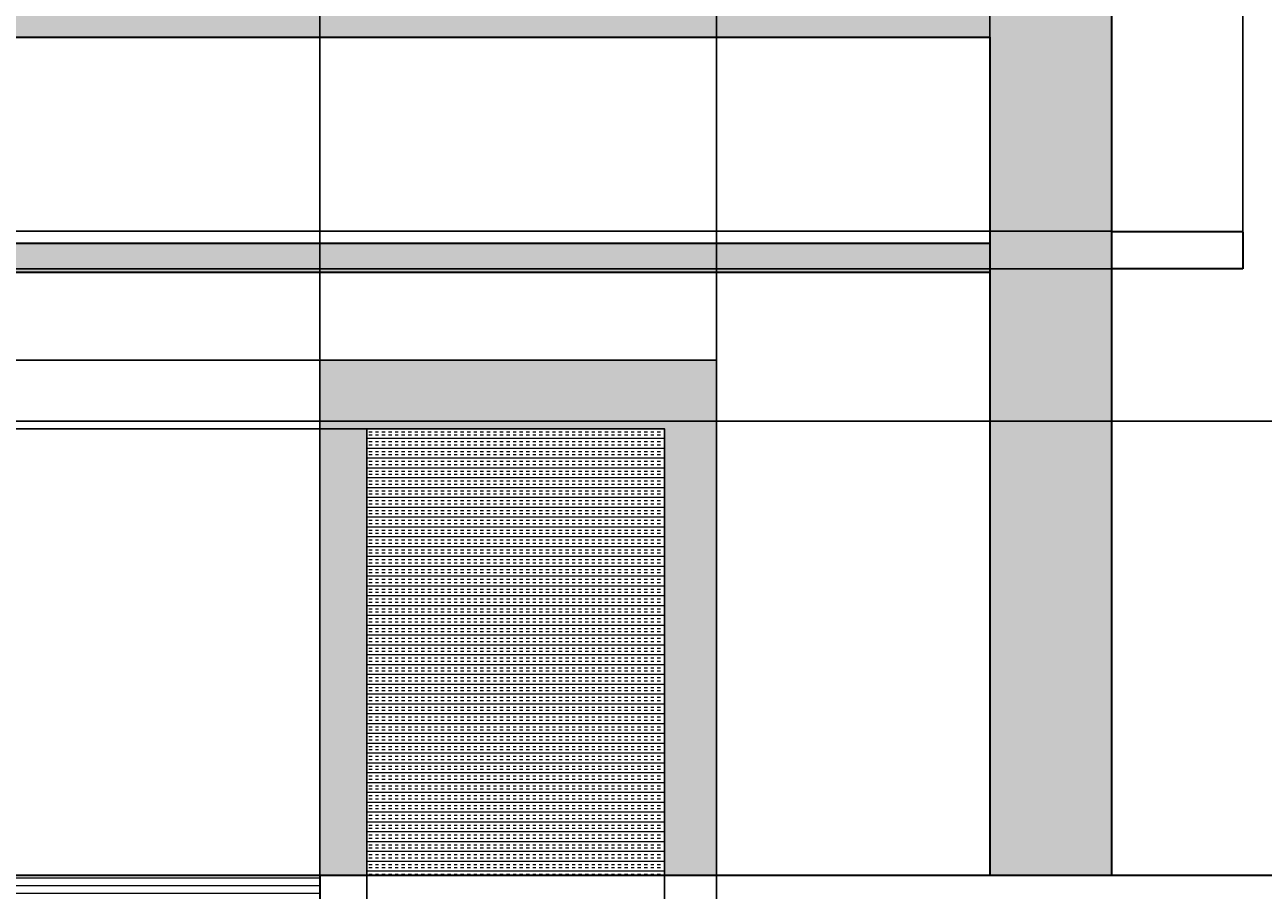
# Model space of a CAD drawing. Units: inches. Extents: x -5 to 714, y 84 to 644.
# Tile 16 of 20: x 457 to 613, y 199 to 308. Entities that reach past the tile are written whole.
import ezdxf

# ---------------------------------------------------------------- set-up
doc = ezdxf.new("R2010")
doc.units = ezdxf.units.IN
doc.header["$MEASUREMENT"] = 0
for name, color, linetype, lineweight in [('A-ANNO-DIMS', 2, 'Continuous', 18), ('A-DOOR', 4, 'Continuous', 25), ('A-ELEV', 7, 'Continuous', 35), ('A-ELEV-PATT', 8, 'Continuous', 13)]:
    doc.layers.add(name, color=color, linetype=linetype, lineweight=lineweight)
doc.styles.get("Standard").update_dxf_attribs({"font": 'arial.ttf'})
doc.dimstyles.get("Standard").update_dxf_attribs({"dimtxt": 0.9375, "dimasz": 0.18, "dimexe": 0.18, "dimexo": 0.0625, "dimgap": 0.09, "dimtad": 0, "dimtih": 1, "dimtoh": 1, "dimdec": 4, "dimzin": 0, "dimdsep": 46, "dimlunit": 4, "dimtxsty": 'Standard', "dimcen": 0.09, "dimadec": 0, "dimazin": 0, "dimtfac": 1, "dimtdec": 4, "dimtofl": 0, "dimtmove": 0, "dimatfit": 3, "dimfxl": 1, "dimtolj": 1, "dimtzin": 0, "dimarcsym": 0})

# ---------------------------------------------------------------- blocks, each defined once
blk = doc.blocks.new('*D55')
at = {"layer": 'A-ANNO-DIMS', "color": 0, "lineweight": -2, "transparency": 16777216}
for p, q in [((593.49, 315.1), (712.66, 315.1)), ((712.48, 314.92), (712.48, 258.71)), ((712.48, 201.37), (712.48, 257.58)), ((593.49, 201.19), (712.66, 201.19))]:
    blk.add_line(p, q, dxfattribs=at)
at = {"layer": 'A-ANNO-DIMS', "color": 0, "transparency": 16777216}
for points in [[(712.45, 314.92), (712.51, 314.92), (712.48, 315.1)], [(712.45, 201.37), (712.51, 201.37), (712.48, 201.19)]]:
    blk.add_solid(points, dxfattribs=at)
at = {"layer": 'Defpoints', "color": 0, "transparency": 16777216}
for p in [(593.43, 315.1), (712.48, 315.1), (593.43, 201.19)]:
    blk.add_point(p, dxfattribs=at)
at = {"layer": 'A-ANNO-DIMS', "color": 0, "transparency": 16777216, "insert": (712.48, 258.14), "char_height": 0.938, "attachment_point": 5}
blk.add_mtext('\\A1;113.9', dxfattribs=at)
blk = doc.blocks.new('*D56')
at = {"layer": 'A-ANNO-DIMS', "color": 0, "lineweight": -2, "transparency": 16777216}
for p, q in [((578.03, 277.05), (-2.74, 277.05)), ((-2.56, 276.87), (-2.56, 239.69)), ((-2.56, 201.37), (-2.56, 238.55)), ((578.03, 201.19), (-2.74, 201.19))]:
    blk.add_line(p, q, dxfattribs=at)
at = {"layer": 'A-ANNO-DIMS', "color": 0, "transparency": 16777216}
for points in [[(-2.59, 276.87), (-2.53, 276.87), (-2.56, 277.05)], [(-2.59, 201.37), (-2.53, 201.37), (-2.56, 201.19)]]:
    blk.add_solid(points, dxfattribs=at)
at = {"layer": 'Defpoints', "color": 0, "transparency": 16777216}
for p in [(-2.56, 277.05), (578.09, 277.05), (578.09, 201.19)]:
    blk.add_point(p, dxfattribs=at)
at = {"layer": 'A-ANNO-DIMS', "color": 0, "transparency": 16777216, "insert": (-2.56, 239.12), "char_height": 0.938, "attachment_point": 5}
blk.add_mtext('\\A1;75.86', dxfattribs=at)
blk = doc.blocks.new('*D57')
at = {"layer": 'A-ANNO-DIMS', "color": 0, "lineweight": -2, "transparency": 16777216}
for p, q in [((578.03, 306.63), (-2.74, 306.63)), ((-2.56, 306.45), (-2.56, 292.41)), ((-2.56, 277.23), (-2.56, 291.27)), ((578.03, 277.05), (-2.74, 277.05))]:
    blk.add_line(p, q, dxfattribs=at)
at = {"layer": 'A-ANNO-DIMS', "color": 0, "transparency": 16777216}
for points in [[(-2.59, 306.45), (-2.53, 306.45), (-2.56, 306.63)], [(-2.59, 277.23), (-2.53, 277.23), (-2.56, 277.05)]]:
    blk.add_solid(points, dxfattribs=at)
at = {"layer": 'Defpoints', "color": 0, "transparency": 16777216}
for p in [(578.09, 306.63), (-2.56, 277.05), (578.09, 277.05)]:
    blk.add_point(p, dxfattribs=at)
at = {"layer": 'A-ANNO-DIMS', "color": 0, "transparency": 16777216, "insert": (-2.56, 291.84), "char_height": 0.938, "attachment_point": 5}
blk.add_mtext('\\A1;29.58', dxfattribs=at)
blk = doc.blocks.new('*D58')
at = {"layer": 'A-ANNO-DIMS', "color": 0, "lineweight": -2, "transparency": 16777216}
for p, q in [((593.43, 282.26), (593.43, 643.61)), ((593.61, 643.43), (600.15, 643.43)), ((609.76, 643.43), (603.22, 643.43)), ((609.94, 282.26), (609.94, 643.61))]:
    blk.add_line(p, q, dxfattribs=at)
at = {"layer": 'A-ANNO-DIMS', "color": 0, "transparency": 16777216}
for points in [[(593.61, 643.46), (593.61, 643.4), (593.43, 643.43)], [(609.76, 643.46), (609.76, 643.4), (609.94, 643.43)]]:
    blk.add_solid(points, dxfattribs=at)
at = {"layer": 'Defpoints', "color": 0, "transparency": 16777216}
for p in [(609.94, 643.43), (593.43, 282.2), (609.94, 282.2)]:
    blk.add_point(p, dxfattribs=at)
at = {"layer": 'A-ANNO-DIMS', "color": 0, "transparency": 16777216, "insert": (601.68, 643.43), "char_height": 0.938, "attachment_point": 5}
blk.add_mtext('\\A1;16.51', dxfattribs=at)
blk = doc.blocks.new('*D59')
at = {"layer": 'A-ANNO-DIMS', "color": 0, "lineweight": -2, "transparency": 16777216}
for p, q in [((593.37, 282.2), (-2.74, 282.2)), ((-2.56, 282.02), (-2.56, 280.41)), ((-2.56, 277.66), (-2.56, 279.27)), ((593.37, 277.48), (-2.74, 277.48))]:
    blk.add_line(p, q, dxfattribs=at)
at = {"layer": 'A-ANNO-DIMS', "color": 0, "transparency": 16777216}
for points in [[(-2.59, 282.02), (-2.53, 282.02), (-2.56, 282.2)], [(-2.59, 277.66), (-2.53, 277.66), (-2.56, 277.48)]]:
    blk.add_solid(points, dxfattribs=at)
at = {"layer": 'Defpoints', "color": 0, "transparency": 16777216}
for p in [(-2.56, 282.2), (593.43, 282.2), (593.43, 277.48)]:
    blk.add_point(p, dxfattribs=at)
at = {"layer": 'A-ANNO-DIMS', "color": 0, "transparency": 16777216, "insert": (-2.56, 279.84), "char_height": 0.938, "attachment_point": 5}
blk.add_mtext('\\A1;4.719', dxfattribs=at)
blk = doc.blocks.new('*D62')
at = {"layer": 'A-ANNO-DIMS', "color": 0, "lineweight": -2, "transparency": 16777216}
for p, q in [((407.38, 266.06), (407.38, 643.61)), ((407.56, 643.43), (449.27, 643.43)), ((493.6, 643.43), (451.89, 643.43)), ((493.78, 266.06), (493.78, 643.61))]:
    blk.add_line(p, q, dxfattribs=at)
at = {"layer": 'A-ANNO-DIMS', "color": 0, "transparency": 16777216}
for points in [[(407.56, 643.46), (407.56, 643.4), (407.38, 643.43)], [(493.6, 643.46), (493.6, 643.4), (493.78, 643.43)]]:
    blk.add_solid(points, dxfattribs=at)
at = {"layer": 'Defpoints', "color": 0, "transparency": 16777216}
for p in [(493.78, 643.43), (407.38, 266), (493.78, 266)]:
    blk.add_point(p, dxfattribs=at)
at = {"layer": 'A-ANNO-DIMS', "color": 0, "transparency": 16777216, "insert": (450.58, 643.43), "char_height": 0.938, "attachment_point": 5}
blk.add_mtext('\\A1;86.4', dxfattribs=at)
blk = doc.blocks.new('*D63')
at = {"layer": 'A-ANNO-DIMS', "color": 0, "lineweight": -2, "transparency": 16777216}
for p, q in [((493.78, 266.06), (493.78, 643.61)), ((493.96, 643.43), (517.06, 643.43)), ((543.54, 643.43), (520.44, 643.43)), ((543.72, 266.06), (543.72, 643.61))]:
    blk.add_line(p, q, dxfattribs=at)
at = {"layer": 'A-ANNO-DIMS', "color": 0, "transparency": 16777216}
for points in [[(493.96, 643.46), (493.96, 643.4), (493.78, 643.43)], [(543.54, 643.46), (543.54, 643.4), (543.72, 643.43)]]:
    blk.add_solid(points, dxfattribs=at)
at = {"layer": 'Defpoints', "color": 0, "transparency": 16777216}
for p in [(543.72, 643.43), (493.78, 266), (543.72, 266)]:
    blk.add_point(p, dxfattribs=at)
at = {"layer": 'A-ANNO-DIMS', "color": 0, "transparency": 16777216, "insert": (518.75, 643.43), "char_height": 0.938, "attachment_point": 5}
blk.add_mtext('\\A1;49.94', dxfattribs=at)
blk = doc.blocks.new('*D64')
at = {"layer": 'A-ANNO-DIMS', "color": 0, "lineweight": -2, "transparency": 16777216}
for p, q in [((543.72, 266.06), (543.72, 643.61)), ((543.9, 643.43), (558.86, 643.43)), ((577.91, 643.43), (562.94, 643.43)), ((578.09, 277.11), (578.09, 643.61))]:
    blk.add_line(p, q, dxfattribs=at)
at = {"layer": 'A-ANNO-DIMS', "color": 0, "transparency": 16777216}
for points in [[(543.9, 643.46), (543.9, 643.4), (543.72, 643.43)], [(577.91, 643.46), (577.91, 643.4), (578.09, 643.43)]]:
    blk.add_solid(points, dxfattribs=at)
at = {"layer": 'Defpoints', "color": 0, "transparency": 16777216}
for p in [(578.09, 643.43), (578.09, 277.05), (543.72, 266)]:
    blk.add_point(p, dxfattribs=at)
at = {"layer": 'A-ANNO-DIMS', "color": 0, "transparency": 16777216, "insert": (560.9, 643.43), "char_height": 0.938, "attachment_point": 5}
blk.add_mtext('\\A1;34.375', dxfattribs=at)
blk = doc.blocks.new('*D69')
at = {"layer": 'A-ANNO-DIMS', "color": 0, "lineweight": -2, "transparency": 16777216}
for p, q in [((403.5, 258.29), (712.66, 258.29)), ((712.48, 258.11), (712.48, 216.52)), ((712.48, 173.8), (712.48, 215.38)), ((403.5, 173.62), (712.66, 173.62))]:
    blk.add_line(p, q, dxfattribs=at)
at = {"layer": 'A-ANNO-DIMS', "color": 0, "transparency": 16777216}
for points in [[(712.45, 258.11), (712.51, 258.11), (712.48, 258.29)], [(712.45, 173.8), (712.51, 173.8), (712.48, 173.62)]]:
    blk.add_solid(points, dxfattribs=at)
at = {"layer": 'Defpoints', "color": 0, "transparency": 16777216}
for p in [(403.44, 258.29), (712.48, 258.29), (403.44, 173.62)]:
    blk.add_point(p, dxfattribs=at)
at = {"layer": 'A-ANNO-DIMS', "color": 0, "transparency": 16777216, "insert": (712.48, 215.95), "char_height": 0.938, "attachment_point": 5}
blk.add_mtext('\\A1;84.67', dxfattribs=at)
blk = doc.blocks.new('*D70')
at = {"layer": 'A-ANNO-DIMS', "color": 0, "lineweight": -2, "transparency": 16777216}
for p, q in [((499.68, 257.28), (499.68, 84.31)), ((537.18, 257.28), (537.18, 84.31)), ((499.86, 84.49), (517.12, 84.49)), ((537, 84.49), (519.74, 84.49))]:
    blk.add_line(p, q, dxfattribs=at)
at = {"layer": 'A-ANNO-DIMS', "color": 0, "transparency": 16777216}
for points in [[(499.86, 84.52), (499.86, 84.46), (499.68, 84.49)], [(537, 84.52), (537, 84.46), (537.18, 84.49)]]:
    blk.add_solid(points, dxfattribs=at)
at = {"layer": 'Defpoints', "color": 0, "transparency": 16777216}
for p in [(499.68, 257.34), (537.18, 257.34), (537.18, 84.49)]:
    blk.add_point(p, dxfattribs=at)
at = {"layer": 'A-ANNO-DIMS', "color": 0, "transparency": 16777216, "insert": (518.43, 84.49), "char_height": 0.938, "attachment_point": 5}
blk.add_mtext('\\A1;37.5', dxfattribs=at)
blk = doc.blocks.new('*D71')
at = {"layer": 'A-ANNO-DIMS', "color": 0, "lineweight": -2, "transparency": 16777216}
for p, q in [((537.12, 257.34), (-2.74, 257.34)), ((-2.56, 257.16), (-2.56, 229.83)), ((-2.56, 201.37), (-2.56, 228.7)), ((537.12, 201.19), (-2.74, 201.19))]:
    blk.add_line(p, q, dxfattribs=at)
at = {"layer": 'A-ANNO-DIMS', "color": 0, "transparency": 16777216}
for points in [[(-2.59, 257.16), (-2.53, 257.16), (-2.56, 257.34)], [(-2.59, 201.37), (-2.53, 201.37), (-2.56, 201.19)]]:
    blk.add_solid(points, dxfattribs=at)
at = {"layer": 'Defpoints', "color": 0, "transparency": 16777216}
for p in [(-2.56, 257.34), (537.18, 257.34), (537.18, 201.19)]:
    blk.add_point(p, dxfattribs=at)
at = {"layer": 'A-ANNO-DIMS', "color": 0, "transparency": 16777216, "insert": (-2.56, 229.27), "char_height": 0.938, "attachment_point": 5}
blk.add_mtext('\\A1;56.15', dxfattribs=at)
blk = doc.blocks.new('*D72')
at = {"layer": 'A-ANNO-DIMS', "color": 0, "lineweight": -2, "transparency": 16777216}
for p, q in [((493.71, 266), (-2.74, 266)), ((-2.56, 265.82), (-2.56, 234.17)), ((-2.56, 201.37), (-2.56, 233.03)), ((493.71, 201.19), (-2.74, 201.19))]:
    blk.add_line(p, q, dxfattribs=at)
at = {"layer": 'A-ANNO-DIMS', "color": 0, "transparency": 16777216}
for points in [[(-2.59, 265.82), (-2.53, 265.82), (-2.56, 266)], [(-2.59, 201.37), (-2.53, 201.37), (-2.56, 201.19)]]:
    blk.add_solid(points, dxfattribs=at)
at = {"layer": 'Defpoints', "color": 0, "transparency": 16777216}
for p in [(-2.56, 266), (493.78, 266), (493.78, 201.19)]:
    blk.add_point(p, dxfattribs=at)
at = {"layer": 'A-ANNO-DIMS', "color": 0, "transparency": 16777216, "insert": (-2.56, 233.6), "char_height": 0.938, "attachment_point": 5}
blk.add_mtext('\\A1;64.81', dxfattribs=at)

msp = doc.modelspace()

# ---------------------------------------------------------------- hatches: boundary and pattern name
at = {"layer": 'A-ELEV-PATT', "transparency": 33554687}
h = msp.add_hatch(color=256, dxfattribs=at)
h.dxf.hatch_style = 1
h.paths.add_polyline_path([(188.3677, 525.1928), (67.9893, 525.1928), (67.9893, 489.1928), (67.9893, 345.1928), (126.7303, 345.1928), (126.7303, 480.1709), (229.3575, 480.1709), (229.3575, 525.1928), (212.6043, 525.1928), (212.6043, 482.7164), (211.0019, 482.7164), (211.0019, 525.1928), (207.6919, 525.1928), (199.9852, 525.1928), (199.9852, 482.7164), (198.3828, 482.7164), (198.3828, 525.1928), (189.9701, 525.1928), (189.9701, 482.7164), (188.3677, 482.7164)])
h.paths.add_polyline_path([(121.3589, 336.2066), (75.5048, 336.2066), (75.5048, 319.345), (121.3589, 319.345)])
h.paths.add_polyline_path([(121.3589, 319.345), (75.5048, 319.345), (75.5048, 302.3045), (121.3589, 302.3045)])
h.paths.add_polyline_path([(121.3589, 302.3045), (75.5048, 302.3045), (75.5048, 282.8561), (121.3589, 282.8561)])
h.paths.add_polyline_path([(121.3589, 282.8561), (75.5048, 282.8561), (75.5048, 261.5556), (121.3589, 261.5556)])
h.paths.add_polyline_path([(121.3589, 261.5556), (75.5048, 261.5556), (75.5048, 243.7009), (121.3589, 243.7009)])
h.paths.add_polyline_path([(121.3589, 243.7009), (75.5048, 243.7009), (75.5048, 223.5117), (121.3589, 223.5117)])
h.paths.add_polyline_path([(121.3589, 223.5117), (75.5048, 223.5117), (75.5048, 212.5836), (121.3589, 212.5836)])
h.paths.add_polyline_path([(121.3589, 212.5836), (75.5048, 212.5836), (75.5048, 201.1928), (121.3589, 201.1928)])
h.paths.add_polyline_path([(179.9335, 201.1928), (30.1395, 201.1928), (30.1395, 198.7054), (179.9335, 198.7054)])
h.paths.add_polyline_path([(187.6349, 201.1928), (179.9335, 201.1928), (179.9335, 198.7054), (179.9335, 141.1928), (269.2446, 141.1928), (269.2446, 201.1928), (263.4349, 201.1928), (263.4349, 152.1176), (187.6349, 152.1176)])
h.paths.add_polyline_path([(269.2446, 277.0513), (269.2446, 287.501), (269.2446, 306.6286), (578.0915, 306.6286), (578.0915, 201.1928), (593.428, 201.1928), (593.428, 315.0968), (584.4202, 315.0968), (259.0665, 315.0968), (259.0665, 201.1928), (263.4349, 201.1928), (269.2446, 201.1928)])
h = msp.add_hatch(color=256, dxfattribs=at)
h.dxf.hatch_style = 1
h.paths.add_polyline_path([(289.8815, 417.0908), (237.2654, 417.0908), (237.2654, 345.1928), (289.8815, 345.1928)])
h.paths.add_polyline_path([(286.8815, 414.0908), (286.8815, 348.1928), (240.2654, 348.1928), (240.2654, 414.0908)], flags=16)
h.paths.add_polyline_path([(244.2856, 376.3091, -1), (241.2767, 376.3091, -1)], flags=0)
h.paths.add_polyline_path([(543.7164, 266.0021), (493.7771, 266.0021), (493.7771, 201.1928), (499.6809, 201.1928), (499.6809, 257.3379), (537.1779, 257.3379), (537.1779, 201.1928), (543.7164, 201.1928)])
h = msp.add_hatch(color=256, dxfattribs=at)
h.dxf.hatch_style = 1
h.paths.add_polyline_path([(578.0915, 280.7123), (269.2446, 280.7123), (269.2446, 277.0513), (578.0915, 277.0513)])
h = msp.add_hatch(color=256, dxfattribs=at)
h.dxf.hatch_style = 1
h.paths.add_polyline_path([(499.6809, 257.3379), (537.1779, 257.3379), (537.1779, 201.1928), (543.7164, 201.1928), (543.7164, 266.0021), (493.7771, 266.0021), (493.7771, 201.1928), (499.6809, 201.1928)])
h.paths.add_polyline_path([(407.3813, 197.3754), (403.4391, 197.3754), (403.4391, 191.3028), (407.3813, 191.3028)])
h.paths.add_polyline_path([(407.3813, 189.3028), (403.4391, 189.3028), (403.4391, 184.8307), (407.3813, 184.8307)])
h.paths.add_polyline_path([(407.3813, 182.8307), (403.4391, 182.8307), (403.4391, 177.6504), (407.3813, 177.6504)])
h.paths.add_polyline_path([(407.3813, 175.6504), (403.4391, 175.6504), (403.4391, 173.6169), (382.4961, 173.6169), (382.4961, 175.6504), (380.7784, 175.6504), (380.7784, 171.1197), (407.3813, 171.1197)])
h.paths.add_polyline_path([(382.4961, 182.8307), (380.7784, 182.8307), (380.7784, 177.6504), (382.4961, 177.6504)])
h.paths.add_polyline_path([(382.4961, 189.3028), (380.7784, 189.3028), (380.7784, 184.8307), (382.4961, 184.8307)])
h.paths.add_polyline_path([(382.4961, 197.3754), (380.7784, 197.3754), (380.7784, 191.3028), (382.4961, 191.3028)])
h.paths.add_polyline_path([(357.6527, 197.3754), (352.9482, 197.3754), (352.9482, 191.3028), (357.6527, 191.3028)])
h.paths.add_polyline_path([(357.6527, 189.3028), (352.9482, 189.3028), (352.9482, 184.8307), (357.6527, 184.8307)])
h.paths.add_polyline_path([(357.6527, 182.8307), (352.9482, 182.8307), (352.9482, 177.6504), (357.6527, 177.6504)])
h.paths.add_polyline_path([(376.2796, 173.6169), (357.6527, 173.6169), (357.6527, 175.6504), (352.9482, 175.6504), (352.9482, 173.6169), (343.9704, 173.6169), (343.9704, 171.1197), (376.2796, 171.1197)])
h.paths.add_polyline_path([(339.2672, 173.6169), (332.0052, 173.6169), (332.0052, 175.6504), (325.8305, 175.6504), (325.8305, 171.1197), (339.2672, 171.1197)])
h.paths.add_polyline_path([(332.0052, 182.8307), (325.8305, 182.8307), (325.8305, 177.6504), (332.0052, 177.6504)])
h.paths.add_polyline_path([(332.0052, 189.3028), (325.8305, 189.3028), (325.8305, 184.8307), (332.0052, 184.8307)])
h.paths.add_polyline_path([(332.0052, 197.3754), (325.8305, 197.3754), (325.8305, 191.3028), (332.0052, 191.3028)])
h = msp.add_hatch(dxfattribs=at)
h.set_pattern_fill('INSUL', color=256, scale=3.3)
h.paths.add_polyline_path([(537.1779, 257.3379), (499.6809, 257.3379), (499.6809, 201.1928), (537.1779, 201.1928)])
h = msp.add_hatch(dxfattribs=at)
h.set_pattern_fill('ANSI31', color=256, scale=7.8, angle=135)
h.paths.add_polyline_path([(493.7771, 201.1928), (454.6437, 201.1928), (454.6437, 141.1928), (493.7771, 141.1928)])
h.paths.add_polyline_path([(489.8003, 196.771), (489.8003, 143.3813), (458.6583, 143.3813), (458.6583, 196.771)], flags=16)

# ---------------------------------------------------------------- linework, layer by layer
at = {"layer": 'A-DOOR'}
for points in [[(493.7771, 266.0021), (543.7164, 266.0021), (543.7164, 158.7212), (493.7771, 158.7212)], [(499.6809, 257.3379), (537.1779, 257.3379), (537.1779, 201.1928), (499.6809, 201.1928)], [(493.7771, 201.1928), (543.7164, 201.1928), (543.7164, 141.1928), (493.7771, 141.1928)]]:
    msp.add_lwpolyline(points, close=True, dxfattribs=at)
at = {"layer": 'A-ELEV'}
for p, q in [((593.428, 315.0968), (593.428, 201.1928)), ((269.2446, 306.6286), (578.0915, 306.6286)), ((578.0915, 306.6286), (578.0915, 201.1928)), ((593.428, 282.1969), (609.9384, 282.1969)), ((609.9384, 282.1969), (609.9384, 277.4776)), ((269.2446, 280.7123), (578.0915, 280.7123)), ((609.9384, 277.4776), (593.428, 277.4776)), ((269.2446, 277.0513), (578.0915, 277.0513)), ((30.1395, 201.1928), (545.1065, 201.1928)), ((493.7771, 201.1928), (493.7771, 141.1928)), ((545.1065, 201.1928), (679.7826, 201.1928))]:
    msp.add_line(p, q, dxfattribs=at)

# ---------------------------------------------------------------- dimensions: what is measured, and where the dimension line sits
at = {"layer": 'A-ANNO-DIMS'}
for base, p1, p2, override, picture, middle in [((493.7771, 643.4276), (407.3813, 266.0021), (493.7771, 266.0021), {"dimdec": 1, "dimlfac": 1, "dimrnd": 0, "dimzin": 0, "dimdsep": 46, "dimlunit": 2}, '*D62', (450.5792, 643.4276)), ((543.7164, 643.4276), (493.7771, 266.0021), (543.7164, 266.0021), {"dimdec": 2, "dimlfac": 1, "dimrnd": 0, "dimzin": 0, "dimdsep": 46, "dimlunit": 2}, '*D63', (518.7468, 643.4276)), ((578.0915, 643.4276), (543.7164, 266.0021), (578.0915, 277.0513), {"dimdec": 3, "dimlfac": 1, "dimrnd": 0, "dimzin": 0, "dimdsep": 46, "dimlunit": 2}, '*D64', (560.904, 643.4276)), ((609.9384, 643.4276), (593.428, 282.1969), (609.9384, 282.1969), {"dimdec": 2, "dimlfac": 1, "dimrnd": 0, "dimzin": 0, "dimdsep": 46, "dimlunit": 2}, '*D58', (601.6832, 643.4276)), ((537.1779, 84.4928), (499.6809, 257.3379), (537.1779, 257.3379), {"dimdec": 1, "dimlfac": 1, "dimrnd": 0, "dimzin": 0, "dimdsep": 46, "dimlunit": 2}, '*D70', (518.4294, 84.4928))]:
    dim = msp.add_linear_dim(base=base, p1=p1, p2=p2, dimstyle='Standard', override=override, dxfattribs=at)
    dim.commit()
    dim.dimension.update_dxf_attribs({"geometry": picture, "text_midpoint": middle})
for base, p1, p2, override, picture, middle in [((712.4826, 315.0968), (593.428, 201.1928), (593.428, 315.0968), {"dimdec": 1, "dimlfac": 1, "dimrnd": 0, "dimzin": 0, "dimdsep": 46, "dimlunit": 2}, '*D55', (712.4826, 258.1448)), ((-2.5605, 277.0513), (578.0915, 306.6286), (578.0915, 277.0513), {"dimdec": 2, "dimlfac": 1, "dimrnd": 0, "dimzin": 0, "dimdsep": 46, "dimlunit": 2}, '*D57', (-2.5605, 291.84)), ((-2.5605, 282.1969), (593.428, 277.4776), (593.428, 282.1969), {"dimdec": 3, "dimlfac": 1, "dimrnd": 0, "dimzin": 0, "dimdsep": 46, "dimlunit": 2}, '*D59', (-2.5605, 279.8372)), ((-2.5605, 277.0513), (578.0915, 201.1928), (578.0915, 277.0513), {"dimdec": 2, "dimlfac": 1, "dimrnd": 0, "dimzin": 0, "dimdsep": 46, "dimlunit": 2}, '*D56', (-2.5605, 239.1221)), ((-2.5605, 266.0021), (493.7771, 201.1928), (493.7771, 266.0021), {"dimdec": 2, "dimlfac": 1, "dimrnd": 0, "dimzin": 0, "dimdsep": 46, "dimlunit": 2}, '*D72', (-2.5605, 233.5974)), ((-2.5605, 257.3379), (537.1779, 201.1928), (537.1779, 257.3379), {"dimdec": 2, "dimlfac": 1, "dimrnd": 0, "dimzin": 0, "dimdsep": 46, "dimlunit": 2}, '*D71', (-2.5605, 229.2653)), ((712.4826, 258.2864), (403.4391, 173.6169), (403.4391, 258.2864), {"dimdec": 2, "dimlfac": 1, "dimrnd": 0, "dimzin": 0, "dimdsep": 46, "dimlunit": 2}, '*D69', (712.4826, 215.9517))]:
    dim = msp.add_linear_dim(base=base, p1=p1, p2=p2, angle=90, dimstyle='Standard', override=override, dxfattribs=at)
    dim.commit()
    dim.dimension.update_dxf_attribs({"geometry": picture, "text_midpoint": middle})

doc.saveas('drawing.dxf')
